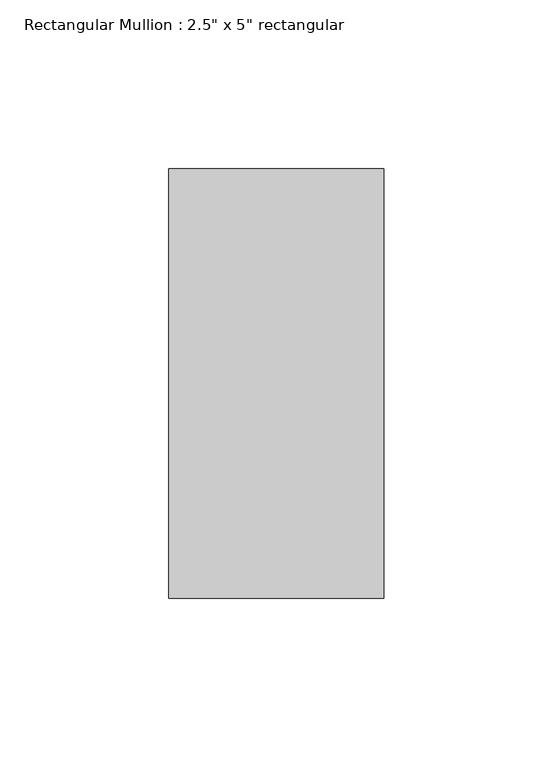
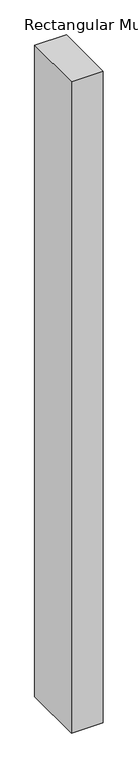
"""IFC4 building model written with IfcOpenShell, lengths in millimetres: member geometry."""

from ifc_helpers import new_model, si_unit, frame, origin, place, context, project, spatial, polyline, outline, extrude, source, transform, mapped, element, save


def member_c31ee173(model_context):
    return source(origin(), model_context, "Body", "SweptSolid", [
        extrude(outline(polyline([(31.75, 63.5), (31.75, -63.5), (-31.75, -63.5), (-31.75, 63.5), (31.75, 63.5)])), frame((0.0, 0.0, -1378.4977008), z_axis=(0.0, 0.0, 1.0), x_axis=(1.0, 0.0, 0.0)), (0.0, 0.0, 1.0), 1378.4977008),
    ])


if __name__ == "__main__":
    model = new_model("IFC4")
    model_context = context("Model", 3, world=origin())
    ifc_project = project(units=[si_unit("LENGTHUNIT", "METRE", prefix="MILLI")], contexts=[model_context])
    site = spatial("IfcSite", under=ifc_project)
    building = spatial("IfcBuilding", under=site)
    placement = place(None, origin())
    member_shape = member_c31ee173(model_context)
    element("IfcMember", 1, ObjectType="Rectangular Mullion : 2.5\" x 5\" rectangular", at=placement, inside=building, context=model_context, shape_type="MappedRepresentation", body=[
        mapped(member_shape, transform((0.0, 0.0, 0.0), x_axis=(1.0, 0.0, 0.0), y_axis=(0.0, 1.0, 0.0), z_axis=(0.0, 0.0, 1.0))),
    ])
    save(model, "model.ifc")

# Revit data of these elements
# Type "Rectangular Mullion : 2.5\" x 5\" rectangular"
#   built-in parameter 1007304 = 0.416667 (stored number, unit not read)
#   built-in parameter 1007301 = 0.104167 (stored number, unit not read)
#   built-in parameter 1007300 = 0.104167 (stored number, unit not read)
# Element 1 (IfcMember, "Rectangular Mullion : 2.5\" x 5\" rectangular")
#   Materials on its faces: "Aluminum"
# Materials
#   "Aluminum": class "Metal", colour RGB 247 247 247, transparency 0, Description = "Aluminum 6061", Cost = 0
